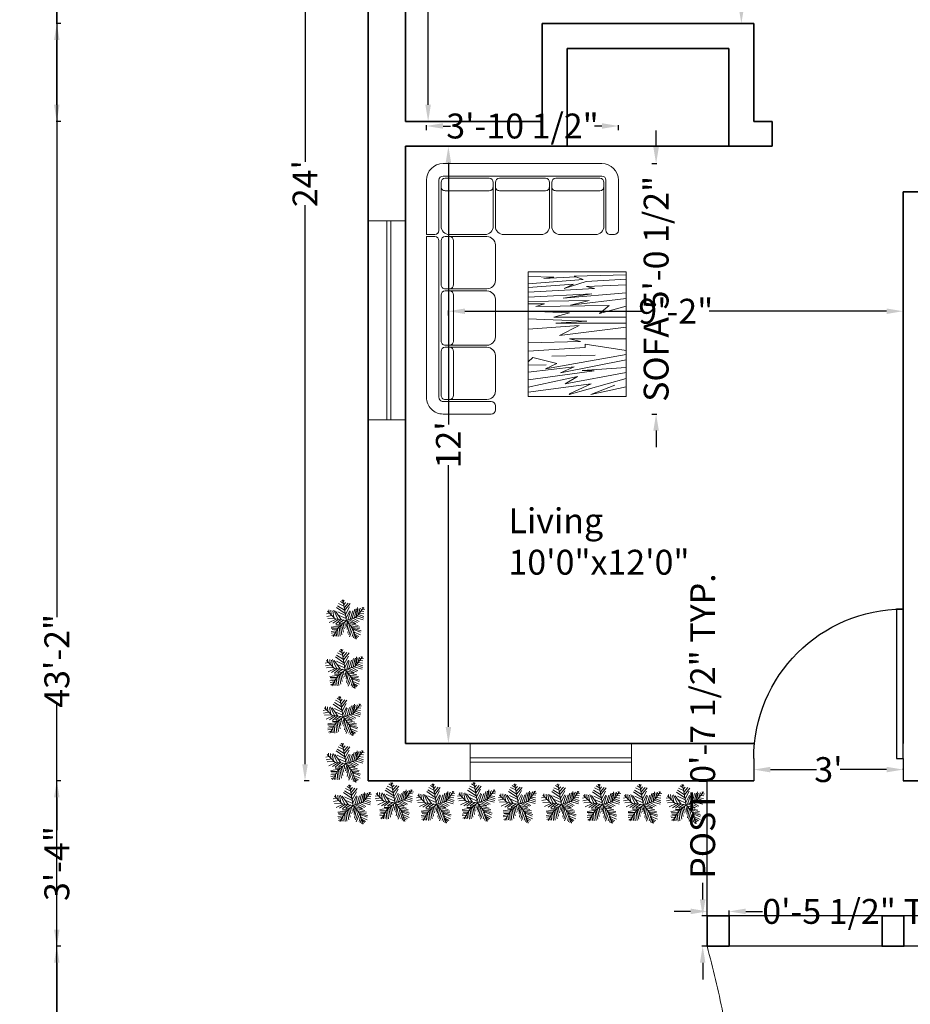
# Model space of a CAD drawing. Units: inches. Extents: x -81 to 380, y -521 to 79.
# Tile 2 of 5: x -81 to 134, y -313 to -76. Entities that reach past the tile are written whole.
import ezdxf

# ---------------------------------------------------------------- set-up
doc = ezdxf.new("R2010")
doc.units = ezdxf.units.IN
doc.header["$MEASUREMENT"] = 0
for name, color, linetype, lineweight in [('A-ANNO-DIMS', 2, 'Continuous', 18), ('A-AREA-IDEN', 5, 'Continuous', 25), ('A-COLS', 34, 'Continuous', 35), ('A-FLOR', 6, 'Continuous', 25), ('A-FURN', 8, 'Continuous', 18), ('A-GLAZ', 4, 'Continuous', 18), ('A-WALL', 249, 'Continuous', 35), ('C-ROAD-DRWY', 6, 'Continuous', 18), ('door', 34, 'Continuous', 25), ('trees', 3, 'Continuous', 13)]:
    doc.layers.add(name, color=color, linetype=linetype, lineweight=lineweight)
doc.styles.get("Standard").update_dxf_attribs({"font": 'arial.ttf'})
doc.dimstyles.get("Standard").update_dxf_attribs({"dimtxt": 6, "dimasz": 4, "dimexe": 0.18, "dimexo": 0.0625, "dimgap": 0.09, "dimtad": 0, "dimdec": 0, "dimzin": 0, "dimdsep": 46, "dimlunit": 3, "dimtxsty": 'Standard', "dimcen": 0.09, "dimclrd": 6, "dimclre": 6, "dimclrt": 2, "dimadec": 0, "dimazin": 0, "dimtfac": 1, "dimtdec": 0, "dimtofl": 0, "dimtmove": 0, "dimatfit": 3, "dimfxl": 1, "dimfxlon": 1, "dimtolj": 1, "dimtzin": 0, "dimarcsym": 0})

# ---------------------------------------------------------------- blocks, each defined once
blk = doc.blocks.new('*U2')
for p, q in [((0, 0), (0, -6)), ((40, 0), (40, -6))]:
    blk.add_line(p, q)
blk.add_lwpolyline([(0, 0), (0, 40), (1.75, 40), (1.75, 0)], close=True)
blk.add_arc((0, 0), 40, 0, 90)
blk = doc.blocks.new('*U4')
for p, q in [((-10.186, 53.64), (-13.084, 55.962)), ((0, 0), (-10.5, 57)), ((-9.099, 51.782), (-6.563, 55.962)), ((-48.585, 21.131), (-49.309, 29.026)), ((-43.513, 28.561), (-42.427, 15.558)), ((-35.544, 28.097), (-24.314, 3.947)), ((-3.665, 19.273), (-27.574, 35.527)), ((-5.114, 28.097), (-24.676, 40.636)), ((-7.288, 39.707), (-21.778, 46.673)), ((-8.737, 47.138), (-17.069, 52.711)), ((-7.65, 43.423), (-2.578, 49.46)), ((-5.839, 35.992), (4.667, 48.067)), ((-5.114, 27.632), (10.463, 46.673)), ((-2.941, 16.486), (8.652, 37.85)), ((16.259, 5.805), (23.142, 31.348)), ((22.055, 7.198), (27.489, 32.277)), ((27, 9), (48, 36)), ((27.127, 9.056), (31.112, 35.992)), ((31.836, 30.883), (32.561, 16.486)), ((35.096, 32.741), (37.27, 22.524)), ((38.719, 34.134), (41.979, 28.561)), ((43.791, 29.954), (51.036, 30.883)), ((44.153, 36.456), (45.239, 32.741)), ((-47.498, 19.737), (-55.83, 18.344)), ((-40.615, 13.7), (-55.105, 10.913)), ((-31.5, 4.5), (-52.5, 25.5)), ((-33.37, 6.269), (-52.207, 5.34)), ((-28.299, 3.483), (-47.86, -5.805)), ((-38.442, 26.239), (-34.819, 7.663)), ((-21.416, 3.018), (-38.079, -8.128)), ((0, 0), (-31.5, 4.5)), ((-14.533, 2.09), (-30.834, 25.31)), ((-15.982, 2.09), (-30.11, -9.521)), ((-24.314, 23.917), (-2.941, 13.7)), ((0, 0), (-22.5, -19.5)), ((-6.563, 1.161), (-21.416, -8.128)), ((-20.691, 13.7), (-1.129, 4.876)), ((-1.129, 6.734), (9.014, 26.704)), ((0, 0), (27, 9)), ((0, 0), (18, -22.5)), ((3.942, 1.625), (11.187, 24.381)), ((6.478, 1.625), (26.04, -8.592)), ((10.101, 3.483), (17.708, 26.239)), ((11.187, 3.483), (30.749, -5.805)), ((18.07, 5.805), (35.096, -3.483)), ((24.229, 7.663), (46.688, 1.625)), ((29.662, 12.307), (48.137, 6.269)), ((33.285, 16.486), (48.862, 10.913)), ((36.183, 19.737), (48.137, 17.88)), ((40.53, 25.775), (48.862, 24.846)), ((-17.431, -15.094), (-42.789, -18.809)), ((-24.314, -21.596), (-42.427, -22.06)), ((-26.849, -26.24), (-40.253, -25.775)), ((-22.5, -19.5), (-37.5, -45)), ((-15.257, -12.772), (-30.11, -12.772)), ((-25.038, -23.918), (-22.865, -45.281)), ((-20.691, -18.345), (-17.793, -44.352)), ((-6.563, -5.805), (-19.967, -9.985)), ((-17.069, -15.094), (-12.721, -40.172)), ((-13.446, -11.378), (-8.737, -32.741)), ((-9.461, -8.592), (-6.201, -23.453)), ((-4.752, -3.483), (-3.665, -14.629)), ((2.493, -3.019), (-1.491, -20.202)), ((1.769, -2.555), (24.229, -9.521)), ((5.029, -6.27), (2.131, -25.775)), ((9.014, -11.378), (3.58, -35.992)), ((14.085, -16.951), (6.478, -40.172)), ((7.565, -9.056), (32.198, -14.629)), ((18.07, -22.524), (8.289, -45.745)), ((12.274, -15.094), (36.907, -18.809)), ((16.259, -19.738), (36.183, -22.989)), ((18, -22.5), (27, -52.5)), ((18.433, -22.524), (40.53, -29.026)), ((19.157, -25.311), (38.719, -33.206)), ((-28.299, -29.026), (-42.789, -31.348)), ((-30.834, -34.135), (-42.427, -35.528)), ((-34.457, -39.708), (-40.978, -42.494)), ((-32.646, -36.921), (-31.921, -44.352)), ((-29.023, -30.884), (-27.936, -43.887)), ((20.244, -30.419), (15.897, -44.816)), ((22.78, -37.85), (19.519, -48.532)), ((21.331, -32.741), (39.081, -40.636)), ((22.78, -38.314), (34.372, -44.816)), ((24.591, -45.745), (23.142, -50.854)), ((24.591, -43.423), (30.749, -47.603)), ((26.764, -49.925), (28.213, -50.854))]:
    blk.add_line(p, q)
blk = doc.blocks.new('*D8')
at = {"layer": 'A-ANNO-DIMS', "color": 0, "lineweight": -2, "transparency": 16777216}
for p, q in [((-10.88, 28.48), (-12.06, 28.48)), ((-11.88, 24.48), (-11.88, -110.29)), ((-11.88, -255.52), (-11.88, -120.75)), ((-10.88, -259.52), (-12.06, -259.52))]:
    blk.add_line(p, q, dxfattribs=at)
at = {"layer": 'A-ANNO-DIMS', "color": 0, "transparency": 16777216}
for points in [[(-12.55, 24.48), (-11.21, 24.48), (-11.88, 28.48)], [(-12.55, -255.52), (-11.21, -255.52), (-11.88, -259.52)]]:
    blk.add_solid(points, dxfattribs=at)
at = {"layer": 'Defpoints', "color": 0, "transparency": 16777216}
for p in [(3.31, 28.48), (-11.88, -259.52), (3.31, -259.52)]:
    blk.add_point(p, dxfattribs=at)
at = {"layer": 'A-ANNO-DIMS', "color": 0, "transparency": 16777216, "insert": (-11.88, -115.52), "char_height": 6, "attachment_point": 5, "rotation": 90}
blk.add_mtext("\\A1;24'", dxfattribs=at)
blk = doc.blocks.new('*D13')
at = {"layer": 'A-ANNO-DIMS', "color": 0, "lineweight": -2, "transparency": 16777216}
for p, q in [((18.8, 19.48), (17.62, 19.48)), ((17.8, 15.48), (17.8, -35.62)), ((17.8, -96.52), (17.8, -45.42)), ((18.8, -100.52), (17.62, -100.52))]:
    blk.add_line(p, q, dxfattribs=at)
at = {"layer": 'A-ANNO-DIMS', "color": 0, "transparency": 16777216}
for points in [[(17.13, 15.48), (18.46, 15.48), (17.8, 19.48)], [(17.13, -96.52), (18.46, -96.52), (17.8, -100.52)]]:
    blk.add_solid(points, dxfattribs=at)
at = {"layer": 'Defpoints', "color": 0, "transparency": 16777216}
for p in [(17.8, 19.48), (28.81, 19.48), (28.81, -100.52)]:
    blk.add_point(p, dxfattribs=at)
at = {"layer": 'A-ANNO-DIMS', "color": 0, "transparency": 16777216, "insert": (17.8, -40.52), "char_height": 6, "attachment_point": 5, "rotation": 90}
blk.add_mtext("\\A1;10'", dxfattribs=at)
blk = doc.blocks.new('*D21')
at = {"layer": 'A-ANNO-DIMS', "color": 0, "lineweight": -2, "transparency": 16777216}
for p, q in [((22.68, -106.52), (22.5, -106.52)), ((22.68, -110.52), (22.68, -173.62)), ((22.68, -246.52), (22.68, -183.42)), ((22.68, -250.52), (22.5, -250.52))]:
    blk.add_line(p, q, dxfattribs=at)
at = {"layer": 'A-ANNO-DIMS', "color": 0, "transparency": 16777216}
for points in [[(22.02, -110.52), (23.35, -110.52), (22.68, -106.52)], [(22.02, -246.52), (23.35, -246.52), (22.68, -250.52)]]:
    blk.add_solid(points, dxfattribs=at)
at = {"layer": 'Defpoints', "color": 0, "transparency": 16777216}
for p in [(22.68, -106.52), (22.68, -106.52), (22.68, -250.52)]:
    blk.add_point(p, dxfattribs=at)
at = {"layer": 'A-ANNO-DIMS', "color": 0, "transparency": 16777216, "insert": (22.68, -178.52), "char_height": 6, "attachment_point": 5, "rotation": 90}
blk.add_mtext("\\A1;12'", dxfattribs=at)
blk = doc.blocks.new('*D22')
at = {"layer": 'A-ANNO-DIMS', "color": 0, "lineweight": -2, "transparency": 16777216}
for p, q in [((22.68, -147.29), (22.68, -146.11)), ((26.68, -146.29), (69.43, -146.29)), ((128.31, -146.29), (85.56, -146.29)), ((132.31, -147.29), (132.31, -146.11))]:
    blk.add_line(p, q, dxfattribs=at)
at = {"layer": 'A-ANNO-DIMS', "color": 0, "transparency": 16777216}
for points in [[(26.68, -145.63), (26.68, -146.96), (22.68, -146.29)], [(128.31, -145.63), (128.31, -146.96), (132.31, -146.29)]]:
    blk.add_solid(points, dxfattribs=at)
at = {"layer": 'Defpoints', "color": 0, "transparency": 16777216}
for p in [(132.31, -146.29), (22.68, -169.26), (132.31, -169.26)]:
    blk.add_point(p, dxfattribs=at)
at = {"layer": 'A-ANNO-DIMS', "color": 0, "transparency": 16777216, "insert": (77.5, -146.29), "char_height": 6, "attachment_point": 5}
blk.add_mtext('\\A1;9\'-2"', dxfattribs=at)
blk = doc.blocks.new('*D23')
at = {"layer": 'A-ANNO-DIMS', "color": 0, "lineweight": -2, "transparency": 16777216}
for p, q in [((96.31, -255.82), (96.31, -257)), ((100.31, -256.82), (111.46, -256.82)), ((128.31, -256.82), (117.16, -256.82)), ((132.31, -256.82), (132.31, -256.64))]:
    blk.add_line(p, q, dxfattribs=at)
at = {"layer": 'A-ANNO-DIMS', "color": 0, "transparency": 16777216}
for points in [[(100.31, -256.15), (100.31, -257.49), (96.31, -256.82)], [(128.31, -256.15), (128.31, -257.49), (132.31, -256.82)]]:
    blk.add_solid(points, dxfattribs=at)
at = {"layer": 'Defpoints', "color": 0, "transparency": 16777216}
for p in [(96.31, -254.12), (132.31, -256.82), (132.31, -256.82)]:
    blk.add_point(p, dxfattribs=at)
at = {"layer": 'A-ANNO-DIMS', "color": 0, "transparency": 16777216, "insert": (114.31, -256.82), "char_height": 6, "attachment_point": 5}
blk.add_mtext("\\A1;3'", dxfattribs=at)
blk = doc.blocks.new('*D28')
at = {"layer": 'A-ANNO-DIMS', "color": 0, "lineweight": -2, "transparency": 16777216}
for p, q in [((92.31, -40.92), (93.49, -40.92)), ((93.31, -44.92), (93.31, -56.07)), ((93.31, -72.92), (93.31, -61.76)), ((92.31, -76.92), (93.49, -76.92))]:
    blk.add_line(p, q, dxfattribs=at)
at = {"layer": 'A-ANNO-DIMS', "color": 0, "transparency": 16777216}
for points in [[(92.64, -44.92), (93.98, -44.92), (93.31, -40.92)], [(92.64, -72.92), (93.98, -72.92), (93.31, -76.92)]]:
    blk.add_solid(points, dxfattribs=at)
at = {"layer": 'Defpoints', "color": 0, "transparency": 16777216}
for p in [(90.31, -40.92), (93.31, -40.92), (90.31, -76.92)]:
    blk.add_point(p, dxfattribs=at)
at = {"layer": 'A-ANNO-DIMS', "color": 0, "transparency": 16777216, "insert": (93.31, -58.92), "char_height": 6, "attachment_point": 5, "rotation": 90}
blk.add_mtext("\\A1;3'", dxfattribs=at)
blk = doc.blocks.new('A$C2AFA021D')
for p, q in [((0.8, 2.3), (0.2, 2.3)), ((0.85, 2.2), (0.85, 2.25)), ((0.2, 2.15), (0.8, 2.15)), ((0.225, 2.125), (0.275, 2.125)), ((0.75, 2.125), (0.275, 2.125)), ((0, 2.1), (0, 0.2)), ((0.15, 0.2), (0.15, 2.1)), ((0.175, 1.55), (0.175, 2.075)), ((0.325, 2.075), (0.325, 1.55)), ((0.85, 1.6), (0.85, 2.025)), ((0.175, 0.875), (0.175, 1.425)), ((0.275, 1.5), (0.225, 1.5)), ((0.225, 1.475), (0.275, 1.475)), ((0.275, 1.5), (0.75, 1.5)), ((0.75, 1.475), (0.275, 1.475)), ((0.325, 1.425), (0.325, 0.875)), ((0.85, 0.925), (0.85, 1.375)), ((0.175, 0.225), (0.175, 0.75)), ((0.275, 0.825), (0.225, 0.825)), ((0.225, 0.8), (0.275, 0.8)), ((0.275, 0.825), (0.75, 0.825)), ((0.75, 0.8), (0.275, 0.8)), ((0.325, 0.75), (0.325, 0.225)), ((0.875, 0.275), (0.875, 0.725)), ((0.975, 0.825), (1.4, 0.825)), ((1.5, 0.725), (1.5, 0.275)), ((1.525, 0.275), (1.525, 0.725)), ((1.625, 0.825), (2.075, 0.825)), ((2.175, 0.725), (2.175, 0.275)), ((2.2, 0.275), (2.2, 0.725)), ((2.3, 0.825), (2.725, 0.825)), ((2.825, 0.725), (2.825, 0.275)), ((2.85, 0.2), (2.85, 0.775)), ((2.9, 0.825), (2.95, 0.825)), ((3, 0.775), (3, 0.2)), ((0.85, 0.275), (0.85, 0.7)), ((0.875, 0.275), (0.875, 0.225)), ((1.45, 0.325), (0.925, 0.325)), ((1.5, 0.225), (1.5, 0.275)), ((1.525, 0.275), (1.525, 0.225)), ((2.125, 0.325), (1.575, 0.325)), ((2.175, 0.225), (2.175, 0.275)), ((2.2, 0.275), (2.2, 0.225)), ((2.775, 0.325), (2.25, 0.325)), ((2.825, 0.225), (2.825, 0.275)), ((0.8, 0.15), (0.2, 0.15)), ((0.275, 0.175), (0.225, 0.175)), ((0.275, 0.175), (0.75, 0.175)), ((0.925, 0.175), (1.45, 0.175)), ((0.925, 0.15), (2.8, 0.15)), ((1.575, 0.175), (2.125, 0.175)), ((2.25, 0.175), (2.775, 0.175)), ((0.85, 0), (0.85, 0.1)), ((0.875, 0.1), (0.875, 0)), ((0.2, 0), (0.85, 0)), ((2.8, 0), (0.875, 0))]:
    blk.add_line(p, q)
for centre, radius, start, end in [((0.2, 2.1), 0.2, 90, 180), ((0.8, 2.25), 0.05, 0, 90), ((0.2, 2.1), 0.05, 90, 180), ((0.225, 2.075), 0.05, 90, 180), ((0.275, 2.075), 0.05, 0, 90), ((0.75, 2.025), 0.1, 0, 90), ((0.8, 2.2), 0.05, 270, 0), ((0.225, 1.55), 0.05, 180, 270), ((0.275, 1.55), 0.05, 270, 0), ((0.75, 1.6), 0.1, 270, 0), ((0.225, 1.425), 0.05, 90, 180), ((0.275, 1.425), 0.05, 0, 90), ((0.75, 1.375), 0.1, 360, 90), ((0.225, 0.875), 0.05, 180, 270), ((0.275, 0.875), 0.05, 270, 0), ((0.75, 0.925), 0.1, 270, 0), ((0.225, 0.75), 0.05, 90, 180), ((0.275, 0.75), 0.05, 0, 90), ((0.75, 0.7), 0.1, 0, 90), ((0.975, 0.725), 0.1, 90, 180), ((1.4, 0.725), 0.1, 0, 90), ((1.625, 0.725), 0.1, 90, 180), ((2.075, 0.725), 0.1, 0, 90), ((2.3, 0.725), 0.1, 90, 180), ((2.725, 0.725), 0.1, 0, 90), ((2.9, 0.775), 0.05, 90, 180), ((2.95, 0.775), 0.05, 0, 90), ((0.75, 0.275), 0.1, 270, 0), ((0.925, 0.275), 0.05, 90, 180), ((1.45, 0.275), 0.05, 360, 90), ((1.575, 0.275), 0.05, 90, 180), ((2.125, 0.275), 0.05, 360, 90), ((2.25, 0.275), 0.05, 90, 180), ((2.775, 0.275), 0.05, 360, 90), ((0.2, 0.2), 0.2, 180, 270), ((0.2, 0.2), 0.05, 180, 270), ((0.225, 0.225), 0.05, 180, 270), ((0.275, 0.225), 0.05, 270, 0), ((0.8, 0.1), 0.05, 0, 90), ((0.925, 0.225), 0.05, 180, 270), ((0.925, 0.1), 0.05, 90, 180), ((1.45, 0.225), 0.05, 270, 0), ((1.575, 0.225), 0.05, 180, 270), ((2.125, 0.225), 0.05, 270, 0), ((2.25, 0.225), 0.05, 180, 270), ((2.775, 0.225), 0.05, 270, 0), ((2.8, 0.2), 0.2, 270, 0), ((2.8, 0.2), 0.05, 270, 0)]:
    blk.add_arc(centre, radius, start, end)
blk = doc.blocks.new('ENTRY-POST')
blk.add_lwpolyline([(0, 7.31), (5.28, 7.31), (5.28, 0), (0, 0)], close=True)
blk = doc.blocks.new('*D38')
at = {"layer": 'A-ANNO-DIMS', "color": 6, "lineweight": -2, "transparency": 16777216}
for p, q in [((83.99, -288.11), (83.99, -284.11)), ((84.99, -292.11), (83.81, -292.11)), ((84.99, -299.41), (83.81, -299.41)), ((83.99, -303.41), (83.99, -307.41))]:
    blk.add_line(p, q, dxfattribs=at)
at = {"layer": 'A-ANNO-DIMS', "color": 6, "transparency": 16777216}
for points in [[(83.32, -288.11), (84.65, -288.11), (83.99, -292.11)], [(83.32, -303.41), (84.65, -303.41), (83.99, -299.41)]]:
    blk.add_solid(points, dxfattribs=at)
at = {"layer": 'Defpoints', "color": 0, "transparency": 16777216}
for p in [(83.99, -292.11), (85.08, -292.11), (85.08, -299.41)]:
    blk.add_point(p, dxfattribs=at)
at = {"layer": 'A-ANNO-DIMS', "color": 2, "transparency": 16777216, "insert": (83.99, -246.31), "char_height": 6, "attachment_point": 5, "rotation": 90}
blk.add_mtext('\\A1;POST 0\'-7 1/2" TYP.', dxfattribs=at)
blk = doc.blocks.new('*D39')
at = {"layer": 'A-ANNO-DIMS', "color": 6, "lineweight": -2, "transparency": 16777216}
for p, q in [((81.08, -291.01), (77.08, -291.01)), ((85.08, -292.01), (85.08, -290.83)), ((90.37, -292.01), (90.37, -290.83)), ((94.37, -291.01), (98.37, -291.01))]:
    blk.add_line(p, q, dxfattribs=at)
at = {"layer": 'A-ANNO-DIMS', "color": 6, "transparency": 16777216}
for points in [[(81.08, -290.34), (81.08, -291.68), (85.08, -291.01)], [(94.37, -290.34), (94.37, -291.68), (90.37, -291.01)]]:
    blk.add_solid(points, dxfattribs=at)
at = {"layer": 'Defpoints', "color": 0, "transparency": 16777216}
for p in [(90.37, -291.01), (85.08, -292.11), (90.37, -292.11)]:
    blk.add_point(p, dxfattribs=at)
at = {"layer": 'A-ANNO-DIMS', "color": 2, "transparency": 16777216, "insert": (123.73, -291.01), "char_height": 6, "attachment_point": 5}
blk.add_mtext('\\A1;0\'-5 1/2" TYP.', dxfattribs=at)
blk = doc.blocks.new('*D42')
at = {"layer": 'A-ANNO-DIMS', "color": 6, "lineweight": -2, "transparency": 16777216}
for p, q in [((72.76, -106.69), (72.76, -102.69)), ((71.76, -110.69), (72.94, -110.69)), ((71.76, -171.09), (72.94, -171.09)), ((72.76, -175.09), (72.76, -179.09))]:
    blk.add_line(p, q, dxfattribs=at)
at = {"layer": 'A-ANNO-DIMS', "color": 6, "transparency": 16777216}
for points in [[(72.09, -106.69), (73.43, -106.69), (72.76, -110.69)], [(72.09, -175.09), (73.43, -175.09), (72.76, -171.09)]]:
    blk.add_solid(points, dxfattribs=at)
at = {"layer": 'Defpoints', "color": 0, "transparency": 16777216}
for p in [(63.7, -110.69), (63.7, -171.09), (72.76, -171.09)]:
    blk.add_point(p, dxfattribs=at)
at = {"layer": 'A-ANNO-DIMS', "color": 2, "transparency": 16777216, "insert": (72.76, -140.89), "char_height": 6, "attachment_point": 5, "rotation": 90}
blk.add_mtext('\\A1;SOFA 5\'-0 1/2"', dxfattribs=at)
blk = doc.blocks.new('*D43')
at = {"layer": 'A-ANNO-DIMS', "color": 6, "lineweight": -2, "transparency": 16777216}
for p, q in [((17.39, -102.63), (17.39, -101.45)), ((21.39, -101.63), (23.16, -101.63)), ((59.7, -101.63), (57.93, -101.63)), ((63.7, -102.63), (63.7, -101.45))]:
    blk.add_line(p, q, dxfattribs=at)
at = {"layer": 'A-ANNO-DIMS', "color": 6, "transparency": 16777216}
for points in [[(21.39, -100.96), (21.39, -102.29), (17.39, -101.63)], [(59.7, -100.96), (59.7, -102.29), (63.7, -101.63)]]:
    blk.add_solid(points, dxfattribs=at)
at = {"layer": 'Defpoints', "color": 0, "transparency": 16777216}
for p in [(63.7, -101.63), (17.39, -110.69), (63.7, -110.69)]:
    blk.add_point(p, dxfattribs=at)
at = {"layer": 'A-ANNO-DIMS', "color": 2, "transparency": 16777216, "insert": (40.55, -101.63), "char_height": 6, "attachment_point": 5}
blk.add_mtext('\\A1;3\'-10 1/2"', dxfattribs=at)
blk = doc.blocks.new('*D46')
at = {"layer": 'A-ANNO-DIMS', "color": 6, "lineweight": -2, "transparency": 16777216}
for p, q in [((74.55, 54.93), (74.55, 56.11)), ((78.55, 55.93), (124.45, 55.93)), ((186.48, 55.93), (140.58, 55.93)), ((190.48, 54.93), (190.48, 56.11))]:
    blk.add_line(p, q, dxfattribs=at)
at = {"layer": 'A-ANNO-DIMS', "color": 6, "transparency": 16777216}
for points in [[(78.55, 56.6), (78.55, 55.26), (74.55, 55.93)], [(186.48, 56.6), (186.48, 55.26), (190.48, 55.93)]]:
    blk.add_solid(points, dxfattribs=at)
at = {"layer": 'Defpoints', "color": 0, "transparency": 16777216}
for p in [(190.48, 55.93), (74.55, -489.67), (190.48, -489.67)]:
    blk.add_point(p, dxfattribs=at)
at = {"layer": 'A-ANNO-DIMS', "color": 2, "transparency": 16777216, "insert": (132.51, 55.93), "char_height": 6, "attachment_point": 5}
blk.add_mtext('\\A1;9\'-8"', dxfattribs=at)
blk = doc.blocks.new('*D47')
at = {"layer": 'A-ANNO-DIMS', "color": 6, "lineweight": -2, "transparency": 16777216}
for p, q in [((-70.72, -299.41), (-71.9, -299.41)), ((-71.72, -303.41), (-71.72, -375.11)), ((-71.72, -485.67), (-71.72, -413.98)), ((-70.72, -489.67), (-71.9, -489.67))]:
    blk.add_line(p, q, dxfattribs=at)
at = {"layer": 'A-ANNO-DIMS', "color": 6, "transparency": 16777216}
for points in [[(-72.39, -303.41), (-71.06, -303.41), (-71.72, -299.41)], [(-72.39, -485.67), (-71.06, -485.67), (-71.72, -489.67)]]:
    blk.add_solid(points, dxfattribs=at)
at = {"layer": 'Defpoints', "color": 0, "transparency": 16777216}
for p in [(-71.72, -299.41), (85.08, -299.41), (74.55, -489.67)]:
    blk.add_point(p, dxfattribs=at)
at = {"layer": 'A-ANNO-DIMS', "color": 2, "transparency": 16777216, "insert": (-71.72, -394.54), "char_height": 6, "attachment_point": 5, "rotation": 90}
blk.add_mtext('\\A1;15\'-10 1/2"', dxfattribs=at)
blk = doc.blocks.new('*D48')
at = {"layer": 'A-ANNO-DIMS', "color": 6, "lineweight": -2, "transparency": 16777216}
for p, q in [((-70.72, 28.48), (-71.9, 28.48)), ((-71.72, 24.48), (-71.72, -220.08)), ((-71.72, -485.67), (-71.72, -241.11)), ((-70.72, -489.67), (-71.9, -489.67))]:
    blk.add_line(p, q, dxfattribs=at)
at = {"layer": 'A-ANNO-DIMS', "color": 6, "transparency": 16777216}
for points in [[(-72.39, 24.48), (-71.06, 24.48), (-71.72, 28.48)], [(-72.39, -485.67), (-71.06, -485.67), (-71.72, -489.67)]]:
    blk.add_solid(points, dxfattribs=at)
at = {"layer": 'Defpoints', "color": 0, "transparency": 16777216}
for p in [(3.31, 28.48), (-71.72, -489.67), (74.55, -489.67)]:
    blk.add_point(p, dxfattribs=at)
at = {"layer": 'A-ANNO-DIMS', "color": 2, "transparency": 16777216, "insert": (-71.72, -230.6), "char_height": 6, "attachment_point": 5, "rotation": 90}
blk.add_mtext('\\A1;43\'-2"', dxfattribs=at)
blk = doc.blocks.new('*D49')
at = {"layer": 'A-ANNO-DIMS', "color": 6, "lineweight": -2, "transparency": 16777216}
for p, q in [((85.08, -516.12), (85.08, -517.3)), ((89.08, -517.12), (122.14, -517.12)), ((175.94, -517.12), (142.88, -517.12)), ((179.94, -516.12), (179.94, -517.3))]:
    blk.add_line(p, q, dxfattribs=at)
at = {"layer": 'A-ANNO-DIMS', "color": 6, "transparency": 16777216}
for points in [[(89.08, -516.45), (89.08, -517.79), (85.08, -517.12)], [(175.94, -516.45), (175.94, -517.79), (179.94, -517.12)]]:
    blk.add_solid(points, dxfattribs=at)
at = {"layer": 'Defpoints', "color": 0, "transparency": 16777216}
for p in [(85.08, -299.41), (179.94, -299.41), (179.94, -517.12)]:
    blk.add_point(p, dxfattribs=at)
at = {"layer": 'A-ANNO-DIMS', "color": 2, "transparency": 16777216, "insert": (132.51, -517.12), "char_height": 6, "attachment_point": 5}
blk.add_mtext('\\A1;7\'-11"', dxfattribs=at)
blk = doc.blocks.new('*D50')
at = {"layer": 'A-ANNO-DIMS', "color": 6, "lineweight": -2, "transparency": 16777216}
for p, q in [((85.08, 54.93), (85.08, 56.11)), ((89.08, 55.93), (98.09, 55.93)), ((123.23, 55.93), (114.22, 55.93)), ((127.23, 54.93), (127.23, 56.11))]:
    blk.add_line(p, q, dxfattribs=at)
at = {"layer": 'A-ANNO-DIMS', "color": 6, "transparency": 16777216}
for points in [[(89.08, 56.6), (89.08, 55.26), (85.08, 55.93)], [(123.23, 56.6), (123.23, 55.26), (127.23, 55.93)]]:
    blk.add_solid(points, dxfattribs=at)
at = {"layer": 'Defpoints', "color": 0, "transparency": 16777216}
for p in [(127.23, 55.93), (85.08, -292.11), (127.23, -292.11)]:
    blk.add_point(p, dxfattribs=at)
at = {"layer": 'A-ANNO-DIMS', "color": 2, "transparency": 16777216, "insert": (106.16, 55.93), "char_height": 6, "attachment_point": 5}
blk.add_mtext('\\A1;3\'-6"', dxfattribs=at)
blk = doc.blocks.new('*D51')
at = {"layer": 'A-ANNO-DIMS', "color": 6, "lineweight": -2, "transparency": 16777216}
for p, q in [((-70.72, -259.52), (-71.9, -259.52)), ((-71.72, -263.52), (-71.72, -271.4)), ((-71.72, -295.41), (-71.72, -287.53)), ((-70.72, -299.41), (-71.9, -299.41))]:
    blk.add_line(p, q, dxfattribs=at)
at = {"layer": 'A-ANNO-DIMS', "color": 6, "transparency": 16777216}
for points in [[(-72.39, -263.52), (-71.06, -263.52), (-71.72, -259.52)], [(-72.39, -295.41), (-71.06, -295.41), (-71.72, -299.41)]]:
    blk.add_solid(points, dxfattribs=at)
at = {"layer": 'Defpoints', "color": 0, "transparency": 16777216}
for p in [(-71.72, -259.52), (85.08, -259.52), (85.08, -299.41)]:
    blk.add_point(p, dxfattribs=at)
at = {"layer": 'A-ANNO-DIMS', "color": 2, "transparency": 16777216, "insert": (-71.72, -279.47), "char_height": 6, "attachment_point": 5, "rotation": 90}
blk.add_mtext('\\A1;3\'-4"', dxfattribs=at)
blk = doc.blocks.new('*D53')
at = {"layer": 'A-ANNO-DIMS', "color": 6, "lineweight": -2, "transparency": 16777216}
for p, q in [((85.08, 54.93), (85.08, 56.11)), ((89.08, 55.93), (92.31, 55.93)), ((96.31, 54.93), (96.31, 56.11)), ((96.31, 55.93), (100.31, 55.93))]:
    blk.add_line(p, q, dxfattribs=at)
at = {"layer": 'A-ANNO-DIMS', "color": 6, "transparency": 16777216}
for points in [[(89.08, 56.6), (89.08, 55.26), (85.08, 55.93)], [(92.31, 56.6), (92.31, 55.26), (96.31, 55.93)]]:
    blk.add_solid(points, dxfattribs=at)
at = {"layer": 'Defpoints', "color": 0, "transparency": 16777216}
for p in [(96.31, 55.93), (85.08, -259.52), (96.31, -259.52)]:
    blk.add_point(p, dxfattribs=at)
at = {"layer": 'A-ANNO-DIMS', "color": 2, "transparency": 16777216, "insert": (110.71, 55.93), "char_height": 6, "attachment_point": 5}
blk.add_mtext('\\A1;0\'-11"', dxfattribs=at)
blk = doc.blocks.new('*D55')
at = {"layer": 'A-ANNO-DIMS', "color": 6, "lineweight": -2, "transparency": 16777216}
for p, q in [((67.53, -517.12), (63.53, -517.12)), ((71.53, -516.12), (71.53, -517.3)), ((90.31, -516.12), (90.31, -517.3)), ((94.31, -517.12), (98.31, -517.12))]:
    blk.add_line(p, q, dxfattribs=at)
at = {"layer": 'A-ANNO-DIMS', "color": 6, "transparency": 16777216}
for points in [[(67.53, -516.45), (67.53, -517.79), (71.53, -517.12)], [(94.31, -516.45), (94.31, -517.79), (90.31, -517.12)]]:
    blk.add_solid(points, dxfattribs=at)
at = {"layer": 'Defpoints', "color": 0, "transparency": 16777216}
for p in [(71.53, -31.92), (90.31, -40.92), (90.31, -517.12)]:
    blk.add_point(p, dxfattribs=at)
at = {"layer": 'A-ANNO-DIMS', "color": 2, "transparency": 16777216, "insert": (80.92, -517.12), "char_height": 6, "attachment_point": 5}
blk.add_mtext('\\A1;1\'-7"', dxfattribs=at)
blk = doc.blocks.new('*D57')
at = {"layer": 'A-ANNO-DIMS', "color": 6, "lineweight": -2, "transparency": 16777216}
for p, q in [((-71.72, -76.92), (-71.72, -72.92)), ((-70.72, -76.92), (-71.9, -76.92)), ((-71.72, -96.52), (-71.72, -80.92)), ((-70.72, -100.52), (-71.9, -100.52))]:
    blk.add_line(p, q, dxfattribs=at)
at = {"layer": 'A-ANNO-DIMS', "color": 6, "transparency": 16777216}
for points in [[(-72.39, -80.92), (-71.06, -80.92), (-71.72, -76.92)], [(-72.39, -96.52), (-71.06, -96.52), (-71.72, -100.52)]]:
    blk.add_solid(points, dxfattribs=at)
at = {"layer": 'Defpoints', "color": 0, "transparency": 16777216}
for p in [(-71.72, -76.92), (45.3, -76.92), (45.3, -100.52)]:
    blk.add_point(p, dxfattribs=at)
at = {"layer": 'A-ANNO-DIMS', "color": 2, "transparency": 16777216, "insert": (-71.72, -55.81), "char_height": 6, "attachment_point": 5, "rotation": 90}
blk.add_mtext('\\A1;1\'-11 1/2"', dxfattribs=at)
blk = doc.blocks.new('*D58')
at = {"layer": 'A-ANNO-DIMS', "color": 6, "lineweight": -2, "transparency": 16777216}
for p, q in [((12.31, -516.12), (12.31, -517.3)), ((16.31, -517.12), (20.69, -517.12)), ((41.3, -517.12), (36.92, -517.12)), ((45.3, -516.12), (45.3, -517.3))]:
    blk.add_line(p, q, dxfattribs=at)
at = {"layer": 'A-ANNO-DIMS', "color": 6, "transparency": 16777216}
for points in [[(16.31, -516.45), (16.31, -517.79), (12.31, -517.12)], [(41.3, -516.45), (41.3, -517.79), (45.3, -517.12)]]:
    blk.add_solid(points, dxfattribs=at)
at = {"layer": 'Defpoints', "color": 0, "transparency": 16777216}
for p in [(12.31, -100.52), (45.3, -100.52), (45.3, -517.12)]:
    blk.add_point(p, dxfattribs=at)
at = {"layer": 'A-ANNO-DIMS', "color": 2, "transparency": 16777216, "insert": (28.81, -517.12), "char_height": 6, "attachment_point": 5}
blk.add_mtext('\\A1;2\'-9"', dxfattribs=at)

msp = doc.modelspace()

# ---------------------------------------------------------------- linework, layer by layer
at = {"layer": 'A-FLOR'}
for p, q in [((85.08, -292.11), (85.08, -259.52)), ((179.94, -292.11), (85.08, -292.11)), ((179.94, -299.41), (85.08, -299.41))]:
    msp.add_line(p, q, dxfattribs=at)
at = {"layer": 'A-FURN'}
for p, q in [((52.98, -137.84), (65.54, -137.49)), ((41.93, -137.94), (48.07, -138.08)), ((41.93, -139.66), (55.18, -138.62)), ((41.93, -140.58), (52.88, -139.79)), ((45.7, -138.38), (53.44, -138)), ((48.07, -138.08), (45.7, -138.38)), ((50.61, -140.79), (55.86, -139.11)), ((52.88, -139.79), (50.61, -140.79)), ((55.18, -138.62), (52.98, -137.84)), ((55.86, -139.11), (65.54, -138.59)), ((65.54, -139.93), (56, -140.34)), ((57.92, -140.85), (41.93, -141.71)), ((41.93, -142.89), (57.27, -142.06)), ((50.37, -143.16), (65.54, -141.89)), ((57.27, -142.06), (50.37, -143.16)), ((56, -140.34), (57.92, -140.85)), ((41.93, -143.92), (56.65, -143.68)), ((41.93, -144.47), (45.84, -144.53)), ((45.84, -144.53), (43.77, -145.19)), ((52.15, -144.81), (65.54, -143.2)), ((56.65, -143.68), (52.15, -144.81)), ((41.93, -146.29), (51.85, -146.67)), ((43.77, -145.19), (61.46, -144.95)), ((51.85, -146.67), (48.07, -147.69)), ((61.46, -144.95), (59.09, -146.87)), ((59.09, -146.87), (65.54, -145.08)), ((41.93, -148.11), (56.04, -148.66)), ((48.07, -147.69), (65.54, -147.69)), ((56.04, -148.66), (48.55, -149.14)), ((48.55, -149.14), (65.54, -149.14)), ((41.93, -150.62), (54.18, -149.73)), ((54.18, -149.73), (49.48, -152.13)), ((49.48, -152.13), (65.54, -150.17)), ((41.93, -153.89), (54.56, -153.58)), ((54.56, -153.58), (51.91, -152.96)), ((51.91, -152.96), (65.54, -152.96)), ((55.69, -155.05), (55.64, -154.25)), ((55.64, -154.25), (65.54, -155.74)), ((41.93, -155.91), (55.69, -155.05)), ((41.93, -158.49), (43.05, -157.42)), ((43.05, -157.42), (48.86, -158.9)), ((46.11, -160.17), (65.54, -156.7)), ((48.86, -158.9), (46.11, -160.17)), ((47.65, -157.12), (58.03, -156.91)), ((49.68, -161.14), (65.54, -157.98)), ((41.93, -159.32), (46.25, -159.18)), ((41.93, -161), (53.01, -159.7)), ((41.93, -162.82), (57.79, -160.69)), ((53.01, -159.7), (49.68, -161.14)), ((50.81, -163.81), (65.54, -161.1)), ((54.94, -160.62), (65.54, -159.9)), ((57.79, -160.69), (54.94, -160.62)), ((41.93, -164.6), (53.84, -162.03)), ((41.93, -165.77), (57.13, -163.81)), ((53.84, -162.03), (50.81, -163.81)), ((51.81, -166.35), (65.54, -162.51)), ((57.13, -163.81), (52.02, -166.11)), ((65.54, -162.51), (65.54, -164.53)), ((52.02, -166.11), (51.81, -166.35)), ((57, -166.39), (62.84, -164.12)), ((65.54, -164.53), (57, -166.39))]:
    msp.add_line(p, q, dxfattribs=at)
msp.add_lwpolyline([(41.93, -136.78), (65.54, -136.78), (65.54, -166.85), (41.93, -166.85)], close=True, dxfattribs=at)
at = {"layer": 'A-GLAZ'}
for p, q in [((12.31, -124.49), (3.31, -124.49)), ((7.81, -124.49), (7.81, -172.49)), ((8.81, -124.49), (8.81, -172.49)), ((12.31, -172.49), (3.31, -172.49)), ((27.93, -250.52), (27.93, -259.52)), ((66.83, -250.69), (66.83, -259.52)), ((27.93, -254.02), (66.83, -254.02)), ((27.93, -255.02), (66.83, -255.02))]:
    msp.add_line(p, q, dxfattribs=at)
at = {"layer": 'A-WALL'}
for p, q in [((3.31, 28.48), (3.31, -259.52)), ((12.31, 19.48), (12.31, -100.52)), ((45.3, -100.52), (45.3, -76.92)), ((45.3, -76.92), (90.31, -76.92)), ((90.31, -76.92), (96.31, -76.92)), ((96.31, -76.92), (96.31, -100.52)), ((51.3, -106.52), (51.3, -82.92)), ((51.3, -82.92), (90.31, -82.92)), ((90.31, -82.92), (90.31, -106.52)), ((12.31, -100.52), (45.3, -100.52)), ((96.31, -100.52), (100.77, -100.52)), ((100.77, -100.52), (100.77, -106.52)), ((12.31, -106.52), (96.31, -106.52)), ((12.31, -106.52), (12.31, -250.52)), ((100.77, -106.52), (96.31, -106.52)), ((132.31, -117.52), (132.31, -250.52)), ((132.31, -117.52), (138.31, -117.52)), ((12.31, -250.52), (96.49, -250.52)), ((3.31, -259.52), (96.31, -259.52)), ((138.31, -259.52), (132.31, -259.52))]:
    msp.add_line(p, q, dxfattribs=at)
at = {"layer": 'C-ROAD-DRWY'}
msp.add_open_spline([(85.08, -299.41), (86.43, -304.77), (92.17, -327.51), (93.95, -372.63), (96.69, -432.53), (81.67, -471.31), (74.55, -489.67)], degree=3, knots=[0, 0, 0, 0, 16.553876, 70.232148, 135.187628, 193.647877, 193.647877, 193.647877, 193.647877], dxfattribs=at)

# ---------------------------------------------------------------- block references
at = {"layer": 'A-COLS'}
for p in [(85.08, -299.41), (127.23, -299.41)]:
    msp.add_blockref('ENTRY-POST', p, dxfattribs=at)
at = {"layer": 'A-FURN', "xscale": 20.13317911396797, "yscale": 20.13317911396797, "zscale": 20.13317911396797, "rotation": 270}
msp.add_blockref('A$C2AFA021D', (17.39, -110.69), dxfattribs=at)
at = {"layer": 'door', "xscale": -0.9, "yscale": 0.9, "zscale": 0.9}
msp.add_blockref('*U2', (132.31, -254.12), dxfattribs=at)
at = {"layer": 'trees', "xscale": 0.0864443764377546, "yscale": 0.0864443764377546, "zscale": 0.0864443764377546}
for p in [(-1.89, -220.84), (-2.17, -232.73), (-2.68, -244.12), (-2, -255.38), (-0.24, -265.44), (9.82, -264.82), (19.83, -265.2), (29.71, -264.83), (39.55, -265.17), (49.99, -265.21), (59.82, -265.26), (69.7, -265.28), (80.02, -265.32)]:
    msp.add_blockref('*U4', p, dxfattribs=at)

# ---------------------------------------------------------------- texts
at = {"layer": 'A-AREA-IDEN', "insert": (37.17, -193.81), "char_height": 6, "attachment_point": 1}
msp.add_mtext_dynamic_manual_height_columns('Living\\P10\'0"x12\'0"', width=81.6384, gutter_width=1, heights=[0], dxfattribs=at)

# ---------------------------------------------------------------- dimensions: what is measured, and where the dimension line sits
at = {"layer": 'A-ANNO-DIMS'}
for base, p1, p2, override, picture, middle in [((190.48, 55.93), (74.55, -489.67), (190.48, -489.67), {"dimdec": 1, "dimlfac": 1, "dimrnd": 0, "dimzin": 1, "dimdsep": 46, "dimlunit": 4, "dimfrac": 2}, '*D46', (132.51, 55.93)), ((127.2309, 55.9306), (85.0832, -292.1074), (127.2309, -292.1074), {"dimdec": 1, "dimlfac": 1, "dimrnd": 0, "dimzin": 1, "dimdsep": 46, "dimlunit": 4, "dimfrac": 2}, '*D50', (106.1571, 55.9306)), ((96.31, 55.93), (85.08, -259.52), (96.31, -259.52), {"dimdec": 1, "dimlfac": 1, "dimrnd": 0, "dimzin": 1, "dimdsep": 46, "dimlunit": 4, "dimfrac": 2}, '*D53', (110.71, 55.93)), ((90.31, -517.12), (71.53, -31.92), (90.31, -40.92), {"dimdec": 1, "dimlfac": 1, "dimrnd": 0, "dimzin": 1, "dimdsep": 46, "dimlunit": 4, "dimfrac": 2}, '*D55', (80.92, -517.12)), ((63.7, -101.63), (17.39, -110.69), (63.7, -110.69), {"dimdec": 1, "dimlfac": 1, "dimrnd": 0, "dimzin": 1, "dimdsep": 46, "dimlunit": 4, "dimfrac": 2}, '*D43', (40.55, -101.63)), ((45.3, -517.12), (12.31, -100.52), (45.3, -100.52), {"dimdec": 1, "dimlfac": 1, "dimrnd": 0, "dimzin": 1, "dimdsep": 46, "dimlunit": 4, "dimfrac": 2}, '*D58', (28.81, -517.12)), ((132.31, -146.29), (22.68, -169.26), (132.31, -169.26), {"dimclrd": 0, "dimclre": 0, "dimclrt": 0}, '*D22', (77.5, -146.29)), ((132.31, -256.82), (96.31, -254.12), (132.31, -256.82), {"dimclrd": 0, "dimclre": 0, "dimclrt": 0}, '*D23', (114.31, -256.82)), ((179.94, -517.12), (85.08, -299.41), (179.94, -299.41), {"dimdec": 1, "dimlfac": 1, "dimrnd": 0, "dimzin": 1, "dimdsep": 46, "dimlunit": 4, "dimfrac": 2}, '*D49', (132.51, -517.12))]:
    dim = msp.add_linear_dim(base=base, p1=p1, p2=p2, dimstyle='Standard', override=override, dxfattribs=at)
    dim.commit()
    dim.dimension.update_dxf_attribs({"geometry": picture, "text_midpoint": middle})
for base, p1, p2, override, picture, middle in [((-71.7227, -489.6708), (3.3113, 28.4806), (74.5527, -489.6708), {"dimdec": 1, "dimlfac": 1, "dimrnd": 0, "dimzin": 1, "dimdsep": 46, "dimlunit": 4, "dimfrac": 2}, '*D48', (-71.7227, -230.5951)), ((-11.88, -259.52), (3.31, 28.48), (3.31, -259.52), {"dimclrd": 0, "dimclre": 0, "dimclrt": 0}, '*D8', (-11.88, -115.52)), ((17.8, 19.48), (28.81, -100.52), (28.81, 19.48), {"dimclrd": 0, "dimclre": 0, "dimclrt": 0}, '*D13', (17.8, -40.52)), ((-71.72, -76.92), (45.3, -100.52), (45.3, -76.92), {"dimdec": 1, "dimlfac": 1, "dimrnd": 0, "dimzin": 1, "dimdsep": 46, "dimlunit": 4, "dimfrac": 2}, '*D57', (-71.72, -55.81)), ((93.31, -40.92), (90.31, -76.92), (90.31, -40.92), {"dimclrd": 0, "dimclre": 0, "dimclrt": 0}, '*D28', (93.31, -58.92)), ((22.68, -106.52), (22.68, -250.52), (22.68, -106.52), {"dimclrd": 0, "dimclre": 0, "dimclrt": 0}, '*D21', (22.68, -178.52)), ((-71.72, -259.52), (85.08, -299.41), (85.08, -259.52), {"dimdec": 1, "dimlfac": 1, "dimrnd": 0, "dimzin": 1, "dimdsep": 46, "dimlunit": 4, "dimfrac": 2}, '*D51', (-71.72, -279.47)), ((-71.72, -299.41), (74.55, -489.67), (85.08, -299.41), {"dimdec": 1, "dimlfac": 1, "dimrnd": 0, "dimzin": 1, "dimdsep": 46, "dimlunit": 4, "dimfrac": 2}, '*D47', (-71.72, -394.54))]:
    dim = msp.add_linear_dim(base=base, p1=p1, p2=p2, angle=90, dimstyle='Standard', override=override, dxfattribs=at)
    dim.commit()
    dim.dimension.update_dxf_attribs({"geometry": picture, "text_midpoint": middle})
for base, p1, p2, angle, text, picture, middle in [((72.76, -171.09), (63.7, -110.69), (63.7, -171.09), 270, 'SOFA <>', '*D42', (72.76, -140.89)), ((83.99, -292.11), (85.08, -299.41), (85.08, -292.11), 90, 'POST <> TYP.', '*D38', (83.99, -246.31))]:
    dim = msp.add_linear_dim(base=base, p1=p1, p2=p2, angle=angle, text=text, dimstyle='Standard', override={"dimdec": 1, "dimlfac": 1, "dimrnd": 0, "dimzin": 1, "dimdsep": 46, "dimlunit": 4, "dimfrac": 2}, dxfattribs=at)
    dim.commit()
    dim.dimension.update_dxf_attribs({"geometry": picture, "text_midpoint": middle})
dim = msp.add_linear_dim(base=(90.37, -291.01), p1=(85.08, -292.11), p2=(90.37, -292.11), text='<> TYP.', dimstyle='Standard', override={"dimdec": 1, "dimlfac": 1, "dimrnd": 0, "dimzin": 1, "dimdsep": 46, "dimlunit": 4, "dimfrac": 2}, dxfattribs=at)
dim.commit()
dim.dimension.update_dxf_attribs({"geometry": '*D39', "text_midpoint": (123.73, -291.01)})

doc.saveas('drawing.dxf')
